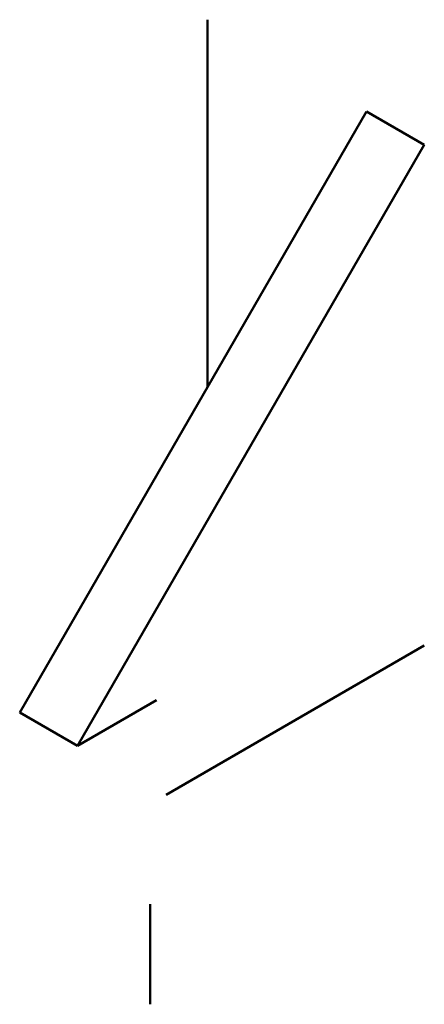
# Model space of a CAD drawing. Units: inches. Extents: x 77 to 4728, y 97 to 6127.
# Tile 2 of 2: x 3496 to 4728, y 3130 to 6127. Entities that reach past the tile are written whole.
import ezdxf

# ---------------------------------------------------------------- set-up
doc = ezdxf.new("R2010")
doc.units = ezdxf.units.IN
doc.header["$MEASUREMENT"] = 0
doc.layers.add('M-OUTL', color=7, linetype='Continuous', lineweight=50)

msp = doc.modelspace()

# ---------------------------------------------------------------- linework, layer by layer
at = {"layer": 'M-OUTL'}
for p, q in [((4068.1, 5009.1), (4068.1, 6126.7)), ((4552.1, 5847.3), (3496.2, 4018.5)), ((4728, 5745.7), (4552.1, 5847.3)), ((4728, 5745.7), (3672.2, 3916.9)), ((3941.8, 3767.8), (4728, 4221.7)), ((3672.2, 3916.9), (3912.4, 4055.6)), ((3672.2, 3916.9), (3496.2, 4018.5)), ((3893.3, 3130.2), (3893.3, 3435))]:
    msp.add_line(p, q, dxfattribs=at)

doc.saveas('drawing.dxf')
